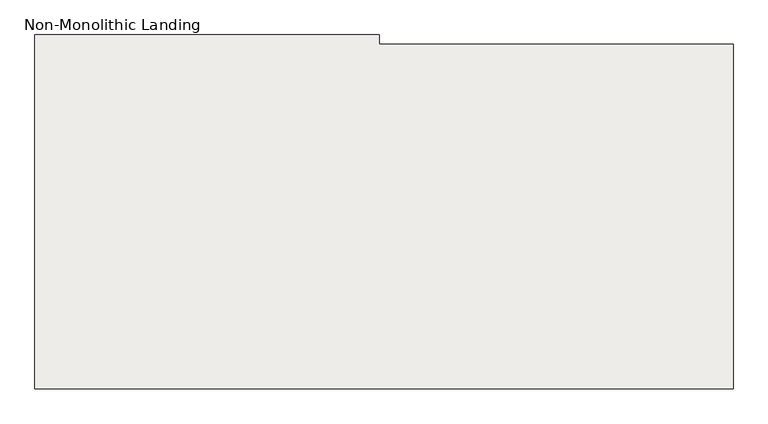
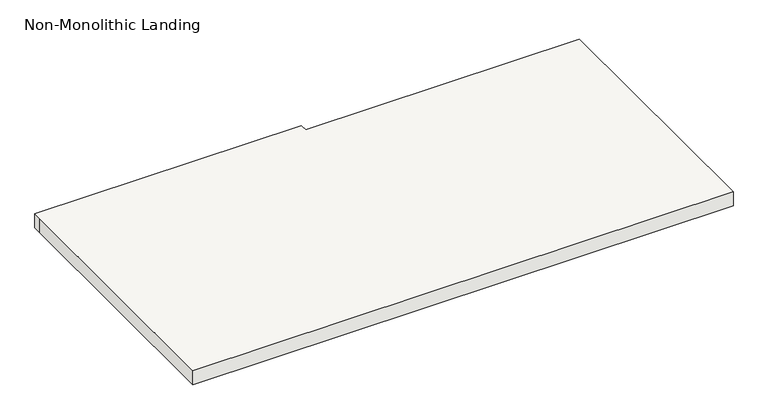
"""IFC4 building model written with IfcOpenShell, lengths in millimetres: slab geometry, Non-Monolithic Landing."""

from ifc_helpers import new_model, si_unit, origin, place, context, project, spatial, faceted_brep, source, transform, mapped, element, save


def non_monolithic_landing_6912f083(model_context):
    return source(origin(), model_context, "Body", "Brep", [
        faceted_brep([(15150.2761273, -3614.7064015, 2368.55), (15150.2761273, -3640.1064015, 2343.15), (14235.8761273, -3640.1064015, 2343.15), (14235.8761273, -3614.7064015, 2368.55), (14210.4761273, -3614.7064015, 2387.6), (14210.4761273, -3589.3064015, 2387.6), (13296.0761273, -3589.3064015, 2387.6), (13296.0761273, -3614.7064015, 2387.6), (13296.0761273, -4529.1064015, 2387.6), (15150.2761273, -4529.1064015, 2387.6), (15150.2761273, -3614.7064015, 2387.6), (14235.8761273, -3640.1064015, 2336.8), (15150.2761273, -3640.1064015, 2336.8), (15150.2761273, -4529.1064015, 2336.8), (13296.0761273, -4529.1064015, 2336.8), (13296.0761273, -3614.7064015, 2336.8), (13296.0761273, -3589.3064015, 2336.8), (14210.4761273, -3589.3064015, 2336.8), (14210.4761273, -3614.7064015, 2336.8), (14235.8761273, -3614.7064015, 2336.8)], [[[0, 1, 2, 3]], [[4, 5, 6, 7, 8, 9, 10]], [[11, 12, 13, 14, 15, 16, 17, 18, 19]], [[12, 11, 2, 1]], [[11, 19, 3, 2]], [[4, 10, 0, 3, 19, 18]], [[5, 4, 18, 17]], [[6, 5, 17, 16]], [[7, 6, 16, 15]], [[8, 7, 15, 14]], [[9, 8, 14, 13]], [[10, 9, 13, 12, 1, 0]]]),
    ])


if __name__ == "__main__":
    model = new_model("IFC4")
    model_context = context("Model", 3, world=origin())
    ifc_project = project(units=[si_unit("LENGTHUNIT", "METRE", prefix="MILLI")], contexts=[model_context])
    site = spatial("IfcSite", under=ifc_project)
    building = spatial("IfcBuilding", under=site)
    placement = place(None, origin())
    non_monolithic_landing_shape = non_monolithic_landing_6912f083(model_context)
    element("IfcSlab", 1, ObjectType="Non-Monolithic Landing", at=placement, inside=building, context=model_context, shape_type="MappedRepresentation", body=[
        mapped(non_monolithic_landing_shape, transform((0.0, 0.0, 0.0), x_axis=(1.0, 0.0, 0.0), y_axis=(0.0, 1.0, 0.0), z_axis=(0.0, 0.0, 1.0))),
    ])
    save(model, "model.ifc")
